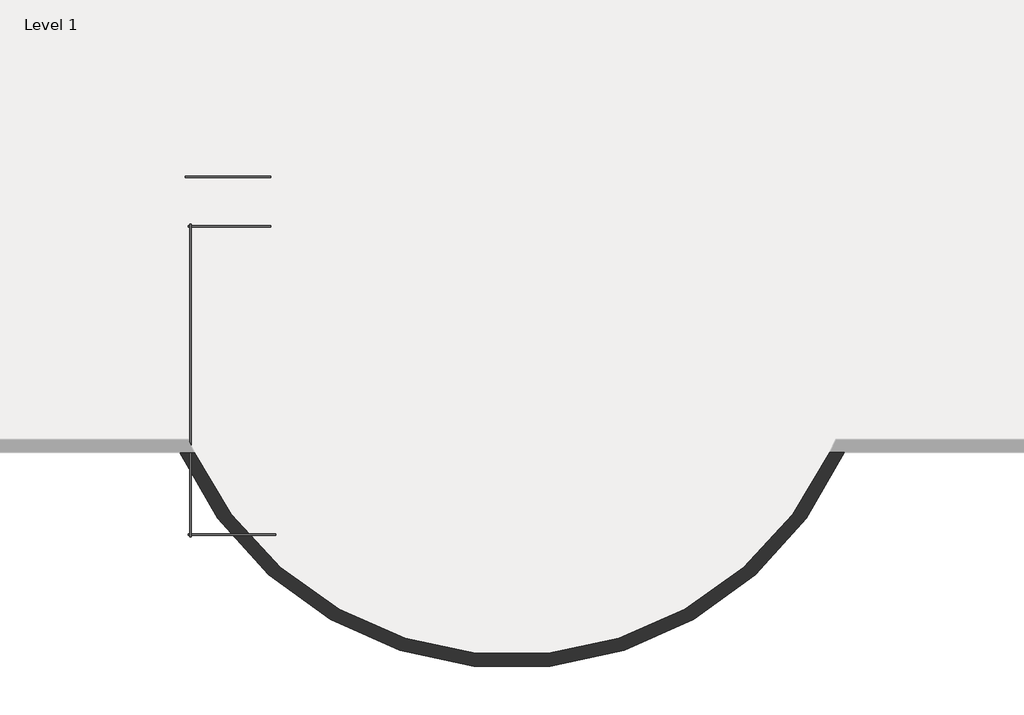
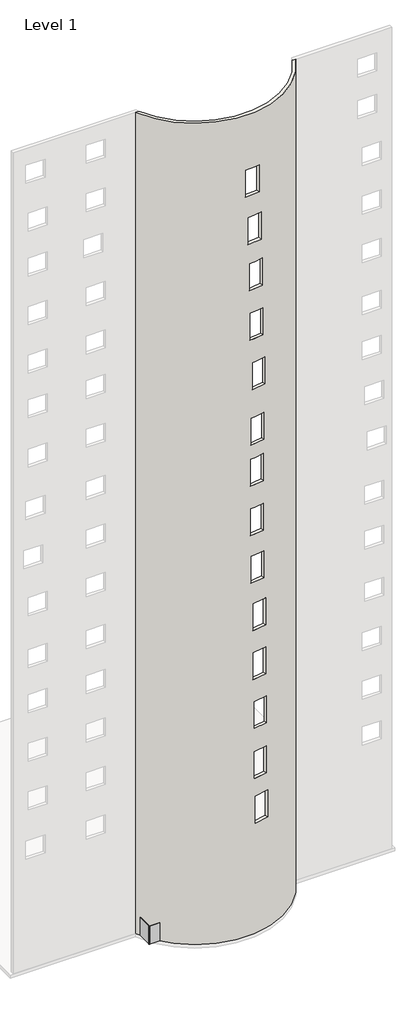
# One storey, part 2 of 3: 4 plates, 1 wall.
"""IFC4 building model written with IfcOpenShell, lengths in millimetres."""

from ifc_helpers import new_model, si_unit, frame, origin, place, context, project, spatial, polyline, circle_curve, transform, mapped, element, save
from ifc_brep_helpers import plane_surface, cylinder_surface, revolved_surface, advanced_brep
from components import system_panel_glazed_7d767388, system_panel_glazed_729cd57b, system_panel_glazed_a9b6887b, system_panel_glazed_c0b1402d

model = new_model("IFC4")

# Units and contexts
model_context = context("Model", 3, world=origin())
ifc_project = project(units=[si_unit("LENGTHUNIT", "METRE", prefix="MILLI")], contexts=[model_context])

# Site, building, storey
site = spatial("IfcSite", under=ifc_project)
building = spatial("IfcBuilding", under=site)
storey = spatial("IfcBuildingStorey", under=building, Name="Level 1", Elevation=0.0)

# Plates
placement = place(None, origin())
system_panel_glazed_shape = system_panel_glazed_7d767388(model_context)
element("IfcPlate", 1, ObjectType="System Panel : Glazed", at=placement, inside=storey, context=model_context, shape_type="MappedRepresentation", body=[
    mapped(system_panel_glazed_shape, transform((-7796.4334489, -15377.6852615, 0.0), x_axis=(1.0, 0.0, 0.0), y_axis=(0.0, 1.0, 0.0), z_axis=(0.0, 0.0, 1.0))),
])
system_panel_glazed_2_shape = system_panel_glazed_729cd57b(model_context)
element("IfcPlate", 2, ObjectType="System Panel : Glazed", at=placement, inside=storey, context=model_context, shape_type="MappedRepresentation", body=[
    mapped(system_panel_glazed_2_shape, transform((-7834.5334489, -10551.6852615, 0.0), x_axis=(-1.0, 0.0, 0.0), y_axis=(0.0, -1.0, 0.0), z_axis=(0.0, 0.0, 1.0))),
])
system_panel_glazed_3_shape = system_panel_glazed_a9b6887b(model_context)
element("IfcPlate", 3, ObjectType="System Panel : Glazed", at=placement, inside=storey, context=model_context, shape_type="MappedRepresentation", body=[
    mapped(system_panel_glazed_3_shape, transform((-7859.9334489, -9789.6852615, 0.0), x_axis=(-1.0, 0.0, 0.0), y_axis=(0.0, -1.0, 0.0), z_axis=(0.0, 0.0, 1.0))),
])
system_panel_glazed_4_shape = system_panel_glazed_c0b1402d(model_context)
element("IfcPlate", 4, ObjectType="System Panel : Glazed", at=placement, inside=storey, context=model_context, shape_type="MappedRepresentation", body=[
    mapped(system_panel_glazed_4_shape, transform((-8469.5334489, -12964.6852615, 0.0), x_axis=(0.0, -1.0, 0.0), y_axis=(1.0, 0.0, 0.0), z_axis=(0.0, 0.0, 1.0))),
])

# Wall
element("IfcWall", 5, ObjectType="Generic - 8\"", at=placement, inside=storey, context=model_context, shape_type="AdvancedBrep", body=[
    advanced_brep(
    [(1429.5064192, -14078.0808221, 55473.6), (-8381.8075047, -14078.0808221, 55473.6), (-8605.1750786, -14078.0808221, 55473.6), (1652.8739931, -14078.0808221, 55473.6), (1429.5064192, -14078.0808221, 0.0), (1652.8739931, -14078.0808221, 0.0), (-8605.1750786, -14078.0808221, 0.0), (-8381.8075047, -14078.0808221, 0.0), (-2594.5712169, -17129.8148783, 51792.5372835), (-3506.1180573, -17201.993253, 51792.5372835), (-3506.1180573, -17201.993253, 49963.7372835), (-2594.5712169, -17129.8148783, 49963.7372835), (-2456.3212223, -17105.1513477, 48533.9772014), (-3365.6892119, -17200.9491525, 48533.9772014), (-3365.6892119, -17200.9491525, 46705.1772014), (-2456.3212223, -17105.1513477, 46705.1772014), (-2361.3526965, -17086.0526721, 45378.432135), (-3268.8610239, -17198.1062109, 45378.432135), (-3268.8610239, -17198.1062109, 43549.632135), (-2361.3526965, -17086.0526721, 43549.632135), (-2331.3322552, -17079.646508, 42011.0775112), (-3238.1906409, -17196.8438988, 42011.0775112), (-3238.1906409, -17196.8438988, 40182.2775112), (-2331.3322552, -17079.646508, 40182.2775112), (-2189.9067254, -17047.0573992, 38624.6599715), (-3093.2976741, -17188.5217194, 38624.6599715), (-3093.2976741, -17188.5217194, 36795.8599715), (-2189.9067254, -17047.0573992, 36795.8599715), (-2256.0685276, -17062.8003995, 34899.6), (-3161.1652841, -17192.9050545, 34899.6), (-3161.1652841, -17192.9050545, 33070.8), (-2256.0685276, -17062.8003995, 33070.8), (-2295.7526892, -17071.8231304, 32142.7093712), (-3201.8019118, -17195.1201953, 32142.7093712), (-3201.8019118, -17195.1201953, 30313.9093712), (-2295.7526892, -17071.8231304, 30313.9093712), (-2304.6906882, -17073.8120688, 28802.2120119), (-3210.9471564, -17195.5764881, 28802.2120119), (-3210.9471564, -17195.5764881, 26973.4120119), (-2304.6906882, -17073.8120688, 26973.4120119), (-2265.1521936, -17064.8933953, 25572.2621165), (-3170.4716309, -17193.4394043, 25572.2621165), (-3170.4716309, -17193.4394043, 23743.4621165), (-2265.1521936, -17064.8933953, 23743.4621165), (-2146.1536843, -17036.1623725, 22324.1324703), (-3048.3350975, -17185.1457865, 22324.1324703), (-3048.3350975, -17185.1457865, 20495.3324703), (-2146.1536843, -17036.1623725, 20495.3324703), (-2135.3051599, -17033.4009928, 19013.8579834), (-3037.1765772, -17184.2496143, 19013.8579834), (-3037.1765772, -17184.2496143, 17185.0579834), (-2135.3051599, -17033.4009928, 17185.0579834), (-2075.3577216, -17017.7099282, 15677.2158009), (-2975.4434279, -17178.8715901, 15677.2158009), (-2975.4434279, -17178.8715901, 13848.4158009), (-2075.3577216, -17017.7099282, 13848.4158009), (-2091.3159895, -17021.9586187, 12298.6447876), (-2991.8891205, -17180.3738824, 12298.6447876), (-2991.8891205, -17180.3738824, 10469.8447876), (-2091.3159895, -17021.9586187, 10469.8447876), (-1978.6055808, -16990.8286463, 9257.587617), (-2875.5472462, -17168.6572404, 9257.587617), (-2875.5472462, -17168.6572404, 7428.787617), (-1978.6055808, -16990.8286463, 7428.787617), (-2578.4761625, -17333.0806904, 51792.5372835), (-2578.4761625, -17333.0806904, 49963.7372835), (-3490.0230029, -17405.2590651, 49963.7372835), (-3490.0230029, -17405.2590651, 51792.5372835), (-2434.9592716, -17307.9312979, 48533.9772014), (-2434.9592716, -17307.9312979, 46705.1772014), (-3344.3272613, -17403.7291027, 46705.1772014), (-3344.3272613, -17403.7291027, 48533.9772014), (-2336.36588, -17288.4179362, 45378.432135), (-2336.36588, -17288.4179362, 43549.632135), (-3243.8742075, -17400.4714751, 43549.632135), (-3243.8742075, -17400.4714751, 45378.432135), (-2305.1984114, -17281.8668417, 42011.0775112), (-2305.1984114, -17281.8668417, 40182.2775112), (-3212.056797, -17399.0642325, 40182.2775112), (-3212.056797, -17399.0642325, 42011.0775112), (-2158.3615994, -17248.5045292, 38624.6599715), (-2158.3615994, -17248.5045292, 36795.8599715), (-3061.7525481, -17389.9688494, 36795.8599715), (-3061.7525481, -17389.9688494, 38624.6599715), (-2227.0564931, -17264.6279076, 34899.6), (-2227.0564931, -17264.6279076, 33070.8), (-3132.1532497, -17394.7325625, 33070.8), (-3132.1532497, -17394.7325625, 34899.6), (-2268.2586791, -17273.8630288, 32142.7093712), (-2268.2586791, -17273.8630288, 30313.9093712), (-3174.3079017, -17397.1600937, 30313.9093712), (-3174.3079017, -17397.1600937, 32142.7093712), (-2277.5384427, -17275.8981809, 28802.2120119), (-2277.5384427, -17275.8981809, 26973.4120119), (-3183.7949109, -17397.6626002, 26973.4120119), (-3183.7949109, -17397.6626002, 28802.2120119), (-2236.4877216, -17266.7705589, 25572.2621165), (-2236.4877216, -17266.7705589, 23743.4621165), (-3141.8071589, -17395.3165679, 23743.4621165), (-3141.8071589, -17395.3165679, 25572.2621165), (-2112.9318757, -17237.3397882, 22324.1324703), (-2112.9318757, -17237.3397882, 20495.3324703), (-3015.113289, -17386.3232022, 20495.3324703), (-3015.113289, -17386.3232022, 22324.1324703), (-2101.6674288, -17234.5092825, 19013.8579834), (-2101.6674288, -17234.5092825, 17185.0579834), (-3003.5388461, -17385.357904, 17185.0579834), (-3003.5388461, -17385.357904, 19013.8579834), (-2039.4202857, -17218.4200222, 15677.2158009), (-2039.4202857, -17218.4200222, 13848.4158009), (-2939.505992, -17379.5816841, 13848.4158009), (-2939.505992, -17379.5816841, 15677.2158009), (-2055.990973, -17222.7774036, 12298.6447876), (-2055.990973, -17222.7774036, 10469.8447876), (-2956.5641039, -17381.1926672, 10469.8447876), (-2956.5641039, -17381.1926672, 12298.6447876), (-1938.9515861, -17190.8376507, 9257.587617), (-1938.9515861, -17190.8376507, 7428.787617), (-2835.8932515, -17368.6662449, 7428.787617), (-2835.8932515, -17368.6662449, 9257.587617)],
    [
        (0, 1, circle_curve(frame((-3476.1505427, -11788.3650223, 55473.6), z_axis=(0.0, 0.0, -1.0), x_axis=(1.0, 0.0, 0.0)), 5413.7111737)),
        (1, 2),
        (2, 3, circle_curve(frame((-3476.1505427, -11788.3650223, 55473.6), z_axis=(0.0, 0.0, 1.0), x_axis=(1.0, 0.0, 0.0)), 5616.9111737)),
        (3, 0),
        (4, 5),
        (5, 6, circle_curve(frame((-3476.1505427, -11788.3650223, 0.0), z_axis=(0.0, 0.0, -1.0), x_axis=(1.0, 0.0, 0.0)), 5616.9111737)),
        (6, 7),
        (7, 4, circle_curve(frame((-3476.1505427, -11788.3650223, 0.0), z_axis=(0.0, 0.0, 1.0), x_axis=(1.0, 0.0, 0.0)), 5413.7111737)),
        (0, 4),
        (7, 1),
        (8, 9, circle_curve(frame((-3476.1505427, -11788.3650223, 51792.5372835), z_axis=(0.0, 0.0, -1.0), x_axis=(1.0, 0.0, 0.0)), 5413.7111737)),
        (9, 10),
        (10, 11, circle_curve(frame((-3476.1505427, -11788.3650223, 49963.7372835), z_axis=(0.0, 0.0, 1.0), x_axis=(1.0, 0.0, 0.0)), 5413.7111737)),
        (11, 8),
        (12, 13, circle_curve(frame((-3476.1505427, -11788.3650223, 48533.9772014), z_axis=(0.0, 0.0, -1.0), x_axis=(1.0, 0.0, 0.0)), 5413.7111737)),
        (13, 14),
        (14, 15, circle_curve(frame((-3476.1505427, -11788.3650223, 46705.1772014), z_axis=(0.0, 0.0, 1.0), x_axis=(1.0, 0.0, 0.0)), 5413.7111737)),
        (15, 12),
        (16, 17, circle_curve(frame((-3476.1505427, -11788.3650223, 45378.432135), z_axis=(0.0, 0.0, -1.0), x_axis=(1.0, 0.0, 0.0)), 5413.7111737)),
        (17, 18),
        (18, 19, circle_curve(frame((-3476.1505427, -11788.3650223, 43549.632135), z_axis=(0.0, 0.0, 1.0), x_axis=(1.0, 0.0, 0.0)), 5413.7111737)),
        (19, 16),
        (20, 21, circle_curve(frame((-3476.1505427, -11788.3650223, 42011.0775112), z_axis=(0.0, 0.0, -1.0), x_axis=(1.0, 0.0, 0.0)), 5413.7111737)),
        (21, 22),
        (22, 23, circle_curve(frame((-3476.1505427, -11788.3650223, 40182.2775112), z_axis=(0.0, 0.0, 1.0), x_axis=(1.0, 0.0, 0.0)), 5413.7111737)),
        (23, 20),
        (24, 25, circle_curve(frame((-3476.1505427, -11788.3650223, 38624.6599715), z_axis=(0.0, 0.0, -1.0), x_axis=(1.0, 0.0, 0.0)), 5413.7111737)),
        (25, 26),
        (26, 27, circle_curve(frame((-3476.1505427, -11788.3650223, 36795.8599715), z_axis=(0.0, 0.0, 1.0), x_axis=(1.0, 0.0, 0.0)), 5413.7111737)),
        (27, 24),
        (28, 29, circle_curve(frame((-3476.1505427, -11788.3650223, 34899.6), z_axis=(0.0, 0.0, -1.0), x_axis=(1.0, 0.0, 0.0)), 5413.7111737)),
        (29, 30),
        (30, 31, circle_curve(frame((-3476.1505427, -11788.3650223, 33070.8), z_axis=(0.0, 0.0, 1.0), x_axis=(1.0, 0.0, 0.0)), 5413.7111737)),
        (31, 28),
        (32, 33, circle_curve(frame((-3476.1505427, -11788.3650223, 32142.7093712), z_axis=(0.0, 0.0, -1.0), x_axis=(1.0, 0.0, 0.0)), 5413.7111737)),
        (33, 34),
        (34, 35, circle_curve(frame((-3476.1505427, -11788.3650223, 30313.9093712), z_axis=(0.0, 0.0, 1.0), x_axis=(1.0, 0.0, 0.0)), 5413.7111737)),
        (35, 32),
        (36, 37, circle_curve(frame((-3476.1505427, -11788.3650223, 28802.2120119), z_axis=(0.0, 0.0, -1.0), x_axis=(1.0, 0.0, 0.0)), 5413.7111737)),
        (37, 38),
        (38, 39, circle_curve(frame((-3476.1505427, -11788.3650223, 26973.4120119), z_axis=(0.0, 0.0, 1.0), x_axis=(1.0, 0.0, 0.0)), 5413.7111737)),
        (39, 36),
        (40, 41, circle_curve(frame((-3476.1505427, -11788.3650223, 25572.2621165), z_axis=(0.0, 0.0, -1.0), x_axis=(1.0, 0.0, 0.0)), 5413.7111737)),
        (41, 42),
        (42, 43, circle_curve(frame((-3476.1505427, -11788.3650223, 23743.4621165), z_axis=(0.0, 0.0, 1.0), x_axis=(1.0, 0.0, 0.0)), 5413.7111737)),
        (43, 40),
        (44, 45, circle_curve(frame((-3476.1505427, -11788.3650223, 22324.1324703), z_axis=(0.0, 0.0, -1.0), x_axis=(1.0, 0.0, 0.0)), 5413.7111737)),
        (45, 46),
        (46, 47, circle_curve(frame((-3476.1505427, -11788.3650223, 20495.3324703), z_axis=(0.0, 0.0, 1.0), x_axis=(1.0, 0.0, 0.0)), 5413.7111737)),
        (47, 44),
        (48, 49, circle_curve(frame((-3476.1505427, -11788.3650223, 19013.8579834), z_axis=(0.0, 0.0, -1.0), x_axis=(1.0, 0.0, 0.0)), 5413.7111737)),
        (49, 50),
        (50, 51, circle_curve(frame((-3476.1505427, -11788.3650223, 17185.0579834), z_axis=(0.0, 0.0, 1.0), x_axis=(1.0, 0.0, 0.0)), 5413.7111737)),
        (51, 48),
        (52, 53, circle_curve(frame((-3476.1505427, -11788.3650223, 15677.2158009), z_axis=(0.0, 0.0, -1.0), x_axis=(1.0, 0.0, 0.0)), 5413.7111737)),
        (53, 54),
        (54, 55, circle_curve(frame((-3476.1505427, -11788.3650223, 13848.4158009), z_axis=(0.0, 0.0, 1.0), x_axis=(1.0, 0.0, 0.0)), 5413.7111737)),
        (55, 52),
        (56, 57, circle_curve(frame((-3476.1505427, -11788.3650223, 12298.6447876), z_axis=(0.0, 0.0, -1.0), x_axis=(1.0, 0.0, 0.0)), 5413.7111737)),
        (57, 58),
        (58, 59, circle_curve(frame((-3476.1505427, -11788.3650223, 10469.8447876), z_axis=(0.0, 0.0, 1.0), x_axis=(1.0, 0.0, 0.0)), 5413.7111737)),
        (59, 56),
        (60, 61, circle_curve(frame((-3476.1505427, -11788.3650223, 9257.587617), z_axis=(0.0, 0.0, -1.0), x_axis=(1.0, 0.0, 0.0)), 5413.7111737)),
        (61, 62),
        (62, 63, circle_curve(frame((-3476.1505427, -11788.3650223, 7428.787617), z_axis=(0.0, 0.0, 1.0), x_axis=(1.0, 0.0, 0.0)), 5413.7111737)),
        (63, 60),
        (2, 6),
        (5, 3),
        (64, 65),
        (65, 66, circle_curve(frame((-3476.1505427, -11788.3650223, 49963.7372835), z_axis=(0.0, 0.0, -1.0), x_axis=(1.0, 0.0, 0.0)), 5616.9111737)),
        (66, 67),
        (67, 64, circle_curve(frame((-3476.1505427, -11788.3650223, 51792.5372835), z_axis=(0.0, 0.0, 1.0), x_axis=(1.0, 0.0, 0.0)), 5616.9111737)),
        (68, 69),
        (69, 70, circle_curve(frame((-3476.1505427, -11788.3650223, 46705.1772014), z_axis=(0.0, 0.0, -1.0), x_axis=(1.0, 0.0, 0.0)), 5616.9111737)),
        (70, 71),
        (71, 68, circle_curve(frame((-3476.1505427, -11788.3650223, 48533.9772014), z_axis=(0.0, 0.0, 1.0), x_axis=(1.0, 0.0, 0.0)), 5616.9111737)),
        (72, 73),
        (73, 74, circle_curve(frame((-3476.1505427, -11788.3650223, 43549.632135), z_axis=(0.0, 0.0, -1.0), x_axis=(1.0, 0.0, 0.0)), 5616.9111737)),
        (74, 75),
        (75, 72, circle_curve(frame((-3476.1505427, -11788.3650223, 45378.432135), z_axis=(0.0, 0.0, 1.0), x_axis=(1.0, 0.0, 0.0)), 5616.9111737)),
        (76, 77),
        (77, 78, circle_curve(frame((-3476.1505427, -11788.3650223, 40182.2775112), z_axis=(0.0, 0.0, -1.0), x_axis=(1.0, 0.0, 0.0)), 5616.9111737)),
        (78, 79),
        (79, 76, circle_curve(frame((-3476.1505427, -11788.3650223, 42011.0775112), z_axis=(0.0, 0.0, 1.0), x_axis=(1.0, 0.0, 0.0)), 5616.9111737)),
        (80, 81),
        (81, 82, circle_curve(frame((-3476.1505427, -11788.3650223, 36795.8599715), z_axis=(0.0, 0.0, -1.0), x_axis=(1.0, 0.0, 0.0)), 5616.9111737)),
        (82, 83),
        (83, 80, circle_curve(frame((-3476.1505427, -11788.3650223, 38624.6599715), z_axis=(0.0, 0.0, 1.0), x_axis=(1.0, 0.0, 0.0)), 5616.9111737)),
        (84, 85),
        (85, 86, circle_curve(frame((-3476.1505427, -11788.3650223, 33070.8), z_axis=(0.0, 0.0, -1.0), x_axis=(1.0, 0.0, 0.0)), 5616.9111737)),
        (86, 87),
        (87, 84, circle_curve(frame((-3476.1505427, -11788.3650223, 34899.6), z_axis=(0.0, 0.0, 1.0), x_axis=(1.0, 0.0, 0.0)), 5616.9111737)),
        (88, 89),
        (89, 90, circle_curve(frame((-3476.1505427, -11788.3650223, 30313.9093712), z_axis=(0.0, 0.0, -1.0), x_axis=(1.0, 0.0, 0.0)), 5616.9111737)),
        (90, 91),
        (91, 88, circle_curve(frame((-3476.1505427, -11788.3650223, 32142.7093712), z_axis=(0.0, 0.0, 1.0), x_axis=(1.0, 0.0, 0.0)), 5616.9111737)),
        (92, 93),
        (93, 94, circle_curve(frame((-3476.1505427, -11788.3650223, 26973.4120119), z_axis=(0.0, 0.0, -1.0), x_axis=(1.0, 0.0, 0.0)), 5616.9111737)),
        (94, 95),
        (95, 92, circle_curve(frame((-3476.1505427, -11788.3650223, 28802.2120119), z_axis=(0.0, 0.0, 1.0), x_axis=(1.0, 0.0, 0.0)), 5616.9111737)),
        (96, 97),
        (97, 98, circle_curve(frame((-3476.1505427, -11788.3650223, 23743.4621165), z_axis=(0.0, 0.0, -1.0), x_axis=(1.0, 0.0, 0.0)), 5616.9111737)),
        (98, 99),
        (99, 96, circle_curve(frame((-3476.1505427, -11788.3650223, 25572.2621165), z_axis=(0.0, 0.0, 1.0), x_axis=(1.0, 0.0, 0.0)), 5616.9111737)),
        (100, 101),
        (101, 102, circle_curve(frame((-3476.1505427, -11788.3650223, 20495.3324703), z_axis=(0.0, 0.0, -1.0), x_axis=(1.0, 0.0, 0.0)), 5616.9111737)),
        (102, 103),
        (103, 100, circle_curve(frame((-3476.1505427, -11788.3650223, 22324.1324703), z_axis=(0.0, 0.0, 1.0), x_axis=(1.0, 0.0, 0.0)), 5616.9111737)),
        (104, 105),
        (105, 106, circle_curve(frame((-3476.1505427, -11788.3650223, 17185.0579834), z_axis=(0.0, 0.0, -1.0), x_axis=(1.0, 0.0, 0.0)), 5616.9111737)),
        (106, 107),
        (107, 104, circle_curve(frame((-3476.1505427, -11788.3650223, 19013.8579834), z_axis=(0.0, 0.0, 1.0), x_axis=(1.0, 0.0, 0.0)), 5616.9111737)),
        (108, 109),
        (109, 110, circle_curve(frame((-3476.1505427, -11788.3650223, 13848.4158009), z_axis=(0.0, 0.0, -1.0), x_axis=(1.0, 0.0, 0.0)), 5616.9111737)),
        (110, 111),
        (111, 108, circle_curve(frame((-3476.1505427, -11788.3650223, 15677.2158009), z_axis=(0.0, 0.0, 1.0), x_axis=(1.0, 0.0, 0.0)), 5616.9111737)),
        (112, 113),
        (113, 114, circle_curve(frame((-3476.1505427, -11788.3650223, 10469.8447876), z_axis=(0.0, 0.0, -1.0), x_axis=(1.0, 0.0, 0.0)), 5616.9111737)),
        (114, 115),
        (115, 112, circle_curve(frame((-3476.1505427, -11788.3650223, 12298.6447876), z_axis=(0.0, 0.0, 1.0), x_axis=(1.0, 0.0, 0.0)), 5616.9111737)),
        (116, 117),
        (117, 118, circle_curve(frame((-3476.1505427, -11788.3650223, 7428.787617), z_axis=(0.0, 0.0, -1.0), x_axis=(1.0, 0.0, 0.0)), 5616.9111737)),
        (118, 119),
        (119, 116, circle_curve(frame((-3476.1505427, -11788.3650223, 9257.587617), z_axis=(0.0, 0.0, 1.0), x_axis=(1.0, 0.0, 0.0)), 5616.9111737)),
        (64, 8),
        (11, 65),
        (10, 66),
        (9, 67),
        (68, 12),
        (15, 69),
        (14, 70),
        (13, 71),
        (72, 16),
        (19, 73),
        (18, 74),
        (17, 75),
        (76, 20),
        (23, 77),
        (22, 78),
        (21, 79),
        (80, 24),
        (27, 81),
        (26, 82),
        (25, 83),
        (84, 28),
        (31, 85),
        (30, 86),
        (29, 87),
        (88, 32),
        (35, 89),
        (34, 90),
        (33, 91),
        (92, 36),
        (39, 93),
        (38, 94),
        (37, 95),
        (96, 40),
        (43, 97),
        (42, 98),
        (41, 99),
        (100, 44),
        (47, 101),
        (46, 102),
        (45, 103),
        (104, 48),
        (51, 105),
        (50, 106),
        (49, 107),
        (108, 52),
        (55, 109),
        (54, 110),
        (53, 111),
        (112, 56),
        (59, 113),
        (58, 114),
        (57, 115),
        (116, 60),
        (63, 117),
        (62, 118),
        (61, 119),
    ],
    [
        plane_surface(frame((1937.560631, -11788.3650223, 55473.6), z_axis=(0.0, 0.0, 1.0), x_axis=(0.0, -1.0, 0.0))),
        plane_surface(frame((1937.560631, -11788.3650223, 0.0), z_axis=(0.0, 0.0, -1.0), x_axis=(0.0, 1.0, 0.0))),
        revolved_surface(polyline([(1937.5606309999994, -11788.3650223, 0.0), (1937.5606309999994, -11788.3650223, 55473.6)]), (-3476.1505427, -11788.3650223, 0.0), (0.0, 0.0, -1.0)),
        cylinder_surface(frame((-3476.1505427, -11788.3650223, 0.0), z_axis=(0.0, 0.0, 1.0), x_axis=(1.0, 0.0, 0.0)), 5616.9111737),
        plane_surface(frame((7877.6494573, -14078.0808221, 0.0), z_axis=(0.0, 1.0, 0.0), x_axis=(1.0, 0.0, 0.0))),
        plane_surface(frame((-16506.3505427, -14078.0808221, 0.0), z_axis=(0.0, 1.0, 0.0), x_axis=(1.0, 0.0, 0.0))),
        plane_surface(frame((-2578.4761625, -17333.0806904, 51792.5372835), z_axis=(-0.9968797467107349, -0.07893523039772028, 0.0), x_axis=(-0.07893523039772028, 0.9968797467107349, 0.0))),
        plane_surface(frame((-2578.4761625, -17333.0806904, 49963.7372835), z_axis=(0.0, 0.0, 1.0), x_axis=(-0.07893523039754888, 0.9968797467107484, 0.0))),
        plane_surface(frame((-3490.0230029, -17405.2590651, 49963.7372835), z_axis=(0.9968797467107351, 0.0789352303977168, 0.0), x_axis=(-0.0789352303977168, 0.9968797467107351, 0.0))),
        plane_surface(frame((-3490.0230029, -17405.2590651, 51792.5372835), z_axis=(0.0, 0.0, -1.0000000000000002), x_axis=(-0.07893523039754528, 0.9968797467107487, 0.0))),
        plane_surface(frame((-2434.9592716, -17307.9312979, 48533.9772014), z_axis=(-0.9944969265536169, -0.10476575335198984, 0.0), x_axis=(-0.10476575335198984, 0.9944969265536169, 0.0))),
        plane_surface(frame((-2434.9592716, -17307.9312979, 46705.1772014), z_axis=(0.0, 0.0, 1.0), x_axis=(-0.10476575335181867, 0.994496926553635, 0.0))),
        plane_surface(frame((-3344.3272613, -17403.7291027, 46705.1772014), z_axis=(0.9944969265536175, 0.10476575335198349, 0.0), x_axis=(-0.10476575335198349, 0.9944969265536175, 0.0))),
        plane_surface(frame((-3344.3272613, -17403.7291027, 48533.9772014), z_axis=(0.0, 0.0, -1.0), x_axis=(-0.10476575335181432, 0.9944969265536354, 0.0))),
        plane_surface(frame((-2336.36588, -17288.4179362, 45378.432135), z_axis=(-0.992463175274333, -0.12254324022315043, 0.0), x_axis=(-0.12254324022315043, 0.992463175274333, 0.0))),
        plane_surface(frame((-2336.36588, -17288.4179362, 43549.632135), z_axis=(0.0, 0.0, 1.0), x_axis=(-0.12254324022298048, 0.9924631752743539, 0.0))),
        plane_surface(frame((-3243.8742075, -17400.4714751, 43549.632135), z_axis=(0.9924631752743326, 0.12254324022315305, 0.0), x_axis=(-0.12254324022315305, 0.9924631752743326, 0.0))),
        plane_surface(frame((-3243.8742075, -17400.4714751, 45378.432135), z_axis=(0.0, 0.0, -1.0), x_axis=(-0.12254324022298303, 0.9924631752743536, 0.0))),
        plane_surface(frame((-2305.1984114, -17281.8668417, 42011.0775112), z_axis=(-0.9917523902379208, -0.12816862508964844, 0.0), x_axis=(-0.12816862508964844, 0.9917523902379208, 0.0))),
        plane_surface(frame((-2305.1984114, -17281.8668417, 40182.2775112), z_axis=(0.0, 0.0, 1.0), x_axis=(-0.128168625089485, 0.9917523902379419, 0.0))),
        plane_surface(frame((-3212.056797, -17399.0642325, 40182.2775112), z_axis=(0.9917523902379202, 0.1281686250896537, 0.0), x_axis=(-0.1281686250896537, 0.9917523902379202, 0.0))),
        plane_surface(frame((-3212.056797, -17399.0642325, 42011.0775112), z_axis=(0.0, 0.0, -1.0), x_axis=(-0.12816862508947735, 0.9917523902379429, 0.0))),
        plane_surface(frame((-2158.3615994, -17248.5045292, 38624.6599715), z_axis=(-0.9879603550433653, -0.15470726182887373, 0.0), x_axis=(-0.15470726182887373, 0.9879603550433653, 0.0))),
        plane_surface(frame((-2158.3615994, -17248.5045292, 36795.8599715), z_axis=(0.0, 0.0, 1.0), x_axis=(-0.15470726182870526, 0.9879603550433916, 0.0))),
        plane_surface(frame((-3061.7525481, -17389.9688494, 36795.8599715), z_axis=(0.987960355043362, 0.15470726182889447, 0.0), x_axis=(-0.15470726182889447, 0.987960355043362, 0.0))),
        plane_surface(frame((-3061.7525481, -17389.9688494, 38624.6599715), z_axis=(0.0, 0.0, -1.0000000000000002), x_axis=(-0.15470726182870365, 0.987960355043392, 0.0))),
        plane_surface(frame((-2227.0564931, -17264.6279076, 34899.6), z_axis=(-0.989825849275452, -0.14228418080071364, 0.0), x_axis=(-0.14228418080071364, 0.989825849275452, 0.0))),
        plane_surface(frame((-2227.0564931, -17264.6279076, 33070.8), z_axis=(0.0, 0.0, 1.0), x_axis=(-0.14228418080055175, 0.9898258492754753, 0.0))),
        plane_surface(frame((-3132.1532497, -17394.7325625, 33070.8), z_axis=(0.9898258492754515, 0.14228418080071753, 0.0), x_axis=(-0.14228418080071753, 0.9898258492754515, 0.0))),
        plane_surface(frame((-3132.1532497, -17394.7325625, 34899.6), z_axis=(0.0, 0.0, -1.0000000000000002), x_axis=(-0.14228418080054955, 0.9898258492754757, 0.0))),
        plane_surface(frame((-2268.2586791, -17273.8630288, 32142.7093712), z_axis=(-0.9908674787839141, -0.1348393098781277, 0.0), x_axis=(-0.1348393098781277, 0.9908674787839141, 0.0))),
        plane_surface(frame((-2268.2586791, -17273.8630288, 30313.9093712), z_axis=(0.0, 0.0, 1.0), x_axis=(-0.13483930987795775, 0.9908674787839371, 0.0))),
        plane_surface(frame((-3174.3079017, -17397.1600937, 30313.9093712), z_axis=(0.990867478783911, 0.13483930987814985, 0.0), x_axis=(-0.13483930987814985, 0.990867478783911, 0.0))),
        plane_surface(frame((-3174.3079017, -17397.1600937, 32142.7093712), z_axis=(0.0, 0.0, -1.0), x_axis=(-0.13483930987795692, 0.9908674787839372, 0.0))),
        plane_surface(frame((-2277.5384427, -17275.8981809, 28802.2120119), z_axis=(-0.9910941253485857, -0.13316318822978884, 0.0), x_axis=(-0.13316318822978884, 0.9910941253485857, 0.0))),
        plane_surface(frame((-2277.5384427, -17275.8981809, 26973.4120119), z_axis=(0.0, 0.0, 1.0000000000000002), x_axis=(-0.13316318822959544, 0.9910941253486116, 0.0))),
        plane_surface(frame((-3183.7949109, -17397.6626002, 26973.4120119), z_axis=(0.9910941253485892, 0.13316318822976145, 0.0), x_axis=(-0.13316318822976145, 0.9910941253485892, 0.0))),
        plane_surface(frame((-3183.7949109, -17397.6626002, 28802.2120119), z_axis=(0.0, 0.0, -1.0), x_axis=(-0.13316318822959172, 0.9910941253486121, 0.0))),
        plane_surface(frame((-2236.4877216, -17266.7705589, 25572.2621165), z_axis=(-0.9900693758779334, -0.14057962494145226, 0.0), x_axis=(-0.14057962494145226, 0.9900693758779334, 0.0))),
        plane_surface(frame((-2236.4877216, -17266.7705589, 23743.4621165), z_axis=(0.0, 0.0, 1.0), x_axis=(-0.14057962494127713, 0.9900693758779583, 0.0))),
        plane_surface(frame((-3141.8071589, -17395.3165679, 23743.4621165), z_axis=(0.9900693758779303, 0.14057962494147438, 0.0), x_axis=(-0.14057962494147438, 0.9900693758779303, 0.0))),
        plane_surface(frame((-3141.8071589, -17395.3165679, 25572.2621165), z_axis=(0.0, 0.0, -1.0000000000000002), x_axis=(-0.1405796249412818, 0.9900693758779577, 0.0))),
        plane_surface(frame((-2112.9318757, -17237.3397882, 22324.1324703), z_axis=(-0.9866375910039811, -0.1629302427969128, 0.0), x_axis=(-0.1629302427969128, 0.9866375910039811, 0.0))),
        plane_surface(frame((-2112.9318757, -17237.3397882, 20495.3324703), z_axis=(0.0, 0.0, 1.0000000000000002), x_axis=(-0.16293024279674612, 0.9866375910040087, 0.0))),
        plane_surface(frame((-3015.113289, -17386.3232022, 20495.3324703), z_axis=(0.9866375910039817, 0.1629302427969089, 0.0), x_axis=(-0.1629302427969089, 0.9866375910039817, 0.0))),
        plane_surface(frame((-3015.113289, -17386.3232022, 22324.1324703), z_axis=(0.0, 0.0, -1.0), x_axis=(-0.1629302427967418, 0.9866375910040094, 0.0))),
        plane_surface(frame((-2101.6674288, -17234.5092825, 19013.8579834), z_axis=(-0.986298575381403, -0.16497005849733762, 0.0), x_axis=(-0.16497005849733762, 0.986298575381403, 0.0))),
        plane_surface(frame((-2101.6674288, -17234.5092825, 17185.0579834), z_axis=(0.0, 0.0, 1.0), x_axis=(-0.16497005849716925, 0.9862985753814311, 0.0))),
        plane_surface(frame((-3003.5388461, -17385.357904, 17185.0579834), z_axis=(0.986298575381403, 0.16497005849733762, 0.0), x_axis=(-0.16497005849733762, 0.986298575381403, 0.0))),
        plane_surface(frame((-3003.5388461, -17385.357904, 19013.8579834), z_axis=(0.0, 0.0, -1.0), x_axis=(-0.16497005849716886, 0.9862985753814312, 0.0))),
        plane_surface(frame((-2039.4202857, -17218.4200222, 15677.2158009), z_axis=(-0.9843456980765554, -0.17624853666961002, 0.0), x_axis=(-0.17624853666961002, 0.9843456980765554, 0.0))),
        plane_surface(frame((-2039.4202857, -17218.4200222, 13848.4158009), z_axis=(0.0, 0.0, 1.0), x_axis=(-0.17624853666944318, 0.9843456980765853, 0.0))),
        plane_surface(frame((-2939.505992, -17379.5816841, 13848.4158009), z_axis=(0.9843456980765559, 0.17624853666960746, 0.0), x_axis=(-0.17624853666960746, 0.9843456980765559, 0.0))),
        plane_surface(frame((-2939.505992, -17379.5816841, 15677.2158009), z_axis=(0.0, 0.0, -1.0), x_axis=(-0.17624853666943913, 0.984345698076586, 0.0))),
        plane_surface(frame((-2055.990973, -17222.7774036, 12298.6447876), z_axis=(-0.9848787521632398, -0.1732450389978875, 0.0), x_axis=(-0.1732450389978875, 0.9848787521632398, 0.0))),
        plane_surface(frame((-2055.990973, -17222.7774036, 10469.8447876), z_axis=(0.0, 0.0, 1.0), x_axis=(-0.1732450389977206, 0.9848787521632693, 0.0))),
        plane_surface(frame((-2956.5641039, -17381.1926672, 10469.8447876), z_axis=(0.9848787521632364, 0.1732450389979076, 0.0), x_axis=(-0.1732450389979076, 0.9848787521632364, 0.0))),
        plane_surface(frame((-2956.5641039, -17381.1926672, 12298.6447876), z_axis=(0.0, 0.0, -1.0), x_axis=(-0.17324503899771596, 0.98487875216327, 0.0))),
        plane_surface(frame((-1938.9515861, -17190.8376507, 9257.587617), z_axis=(-0.9809073331069991, -0.19447571533976912, 0.0), x_axis=(-0.19447571533976912, 0.9809073331069991, 0.0))),
        plane_surface(frame((-1938.9515861, -17190.8376507, 7428.787617), z_axis=(0.0, 0.0, 1.0), x_axis=(-0.19447571533960262, 0.980907333107032, 0.0))),
        plane_surface(frame((-2835.8932515, -17368.6662449, 7428.787617), z_axis=(0.9809073331069983, 0.19447571533977293, 0.0), x_axis=(-0.19447571533977293, 0.9809073331069983, 0.0))),
        plane_surface(frame((-2835.8932515, -17368.6662449, 9257.587617), z_axis=(0.0, 0.0, -1.0), x_axis=(-0.1944757153395977, 0.980907333107033, 0.0))),
    ],
    [
        (0, [[1, 2, 3, 4]]),
        (1, [[5, 6, 7, 8]]),
        (2, [[-1, 9, -8, 10], [11, 12, 13, 14], [15, 16, 17, 18], [19, 20, 21, 22], [23, 24, 25, 26], [27, 28, 29, 30], [31, 32, 33, 34], [35, 36, 37, 38], [39, 40, 41, 42], [43, 44, 45, 46], [47, 48, 49, 50], [51, 52, 53, 54], [55, 56, 57, 58], [59, 60, 61, 62], [63, 64, 65, 66]]),
        (3, [[-3, 67, -6, 68], [69, 70, 71, 72], [73, 74, 75, 76], [77, 78, 79, 80], [81, 82, 83, 84], [85, 86, 87, 88], [89, 90, 91, 92], [93, 94, 95, 96], [97, 98, 99, 100], [101, 102, 103, 104], [105, 106, 107, 108], [109, 110, 111, 112], [113, 114, 115, 116], [117, 118, 119, 120], [121, 122, 123, 124]]),
        (4, [[-4, -68, -5, -9]]),
        (5, [[-2, -10, -7, -67]]),
        (6, [[-69, 125, -14, 126]]),
        (7, [[-70, -126, -13, 127]]),
        (8, [[-71, -127, -12, 128]]),
        (9, [[-72, -128, -11, -125]]),
        (10, [[-73, 129, -18, 130]]),
        (11, [[-74, -130, -17, 131]]),
        (12, [[-75, -131, -16, 132]]),
        (13, [[-76, -132, -15, -129]]),
        (14, [[-77, 133, -22, 134]]),
        (15, [[-78, -134, -21, 135]]),
        (16, [[-79, -135, -20, 136]]),
        (17, [[-80, -136, -19, -133]]),
        (18, [[-81, 137, -26, 138]]),
        (19, [[-82, -138, -25, 139]]),
        (20, [[-83, -139, -24, 140]]),
        (21, [[-84, -140, -23, -137]]),
        (22, [[-85, 141, -30, 142]]),
        (23, [[-86, -142, -29, 143]]),
        (24, [[-87, -143, -28, 144]]),
        (25, [[-88, -144, -27, -141]]),
        (26, [[-89, 145, -34, 146]]),
        (27, [[-90, -146, -33, 147]]),
        (28, [[-91, -147, -32, 148]]),
        (29, [[-92, -148, -31, -145]]),
        (30, [[-93, 149, -38, 150]]),
        (31, [[-94, -150, -37, 151]]),
        (32, [[-95, -151, -36, 152]]),
        (33, [[-96, -152, -35, -149]]),
        (34, [[-97, 153, -42, 154]]),
        (35, [[-98, -154, -41, 155]]),
        (36, [[-99, -155, -40, 156]]),
        (37, [[-100, -156, -39, -153]]),
        (38, [[-101, 157, -46, 158]]),
        (39, [[-102, -158, -45, 159]]),
        (40, [[-103, -159, -44, 160]]),
        (41, [[-104, -160, -43, -157]]),
        (42, [[-105, 161, -50, 162]]),
        (43, [[-106, -162, -49, 163]]),
        (44, [[-107, -163, -48, 164]]),
        (45, [[-108, -164, -47, -161]]),
        (46, [[-109, 165, -54, 166]]),
        (47, [[-110, -166, -53, 167]]),
        (48, [[-111, -167, -52, 168]]),
        (49, [[-112, -168, -51, -165]]),
        (50, [[-113, 169, -58, 170]]),
        (51, [[-114, -170, -57, 171]]),
        (52, [[-115, -171, -56, 172]]),
        (53, [[-116, -172, -55, -169]]),
        (54, [[-117, 173, -62, 174]]),
        (55, [[-118, -174, -61, 175]]),
        (56, [[-119, -175, -60, 176]]),
        (57, [[-120, -176, -59, -173]]),
        (58, [[-121, 177, -66, 178]]),
        (59, [[-122, -178, -65, 179]]),
        (60, [[-123, -179, -64, 180]]),
        (61, [[-124, -180, -63, -177]]),
    ],
),
])

save(model, "model.ifc")

# Revit data of these elements
# Type "System Panel : Glazed"
#   Construction Type Id = "GSP4R"
#   Analytic Construction = "1/8 in Pilkington single glazing"
#   Visual Light Transmittance = 0.9
#   Solar Heat Gain Coefficient = 0.86
#   Heat Transfer Coefficient (U) = 1.18115 BTU/(h·ft²·°F)
# Type "Generic - 8\""
#   Assembly Code = "B2010"
#   Layers, outside or top first: 0' - 8" no material (function 1)
# Elements 1, 2, 3, 4 (IfcPlate, "System Panel : Glazed")
#   Phase Created = New Construction
#   Materials on its faces: "Glass"
# Element 5 (IfcWall, "Generic - 8\"")
#   Top Offset = 0' - 0"
#   Base Offset = 0' - 0"
#   Unconnected Height = 182' - 0"
#   wall height = 182' - 0"
#   Phase Created = New Construction
#   Materials on its faces: "Default Wall"
# Materials
#   "Glass": class "Glass", colour RGB 0 128 192, transparency 0.75, Description = "Soda Lime Glass", Cost = 0
#   "Default Wall": colour RGB 128 128 128, transparency 0
